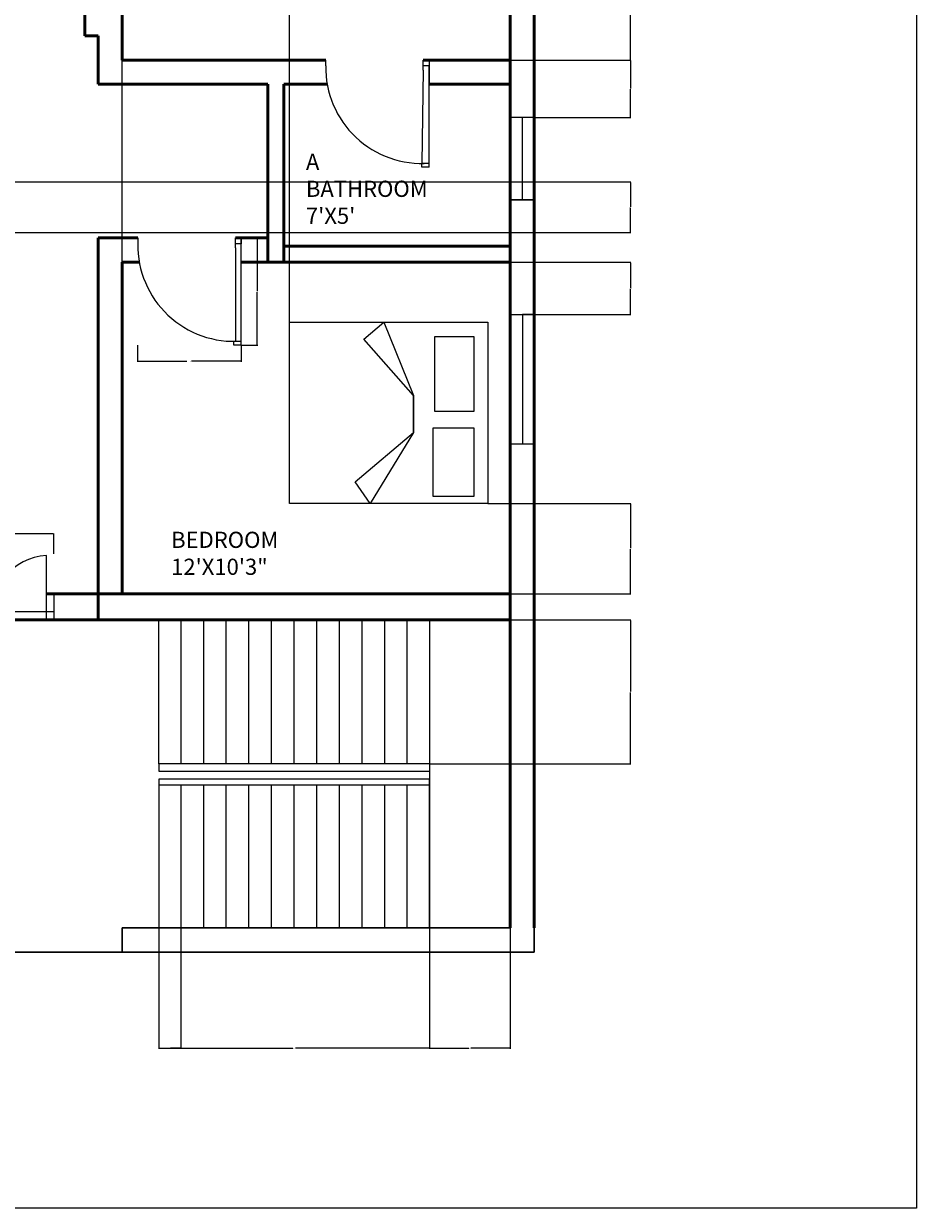
# Model space of a CAD drawing. Units: inches. Extents: x -177 to 2564, y -706 to 2548.
# Tile 2 of 4: x 192 to 523, y -706 to -266. Entities that reach past the tile are written whole.
import ezdxf

# ---------------------------------------------------------------- set-up
doc = ezdxf.new("R2010")
doc.units = ezdxf.units.IN
doc.header["$MEASUREMENT"] = 0
for name, color, linetype, lineweight in [('A-ANNO-DIMS', 2, 'Continuous', 18), ('A-ANNO-TTLB', 7, 'Continuous', 25), ('A-AREA-IDEN', 7, 'Continuous', 25), ('A-DOOR', 3, 'Continuous', 25), ('A-FLOR-OTLN', 7, 'Continuous', 30), ('A-FLOR-STRS', 6, 'Continuous', 25), ('A-FURN', 8, 'Continuous', 18), ('A-GLAZ', 4, 'Continuous', 18), ('A-WALL', 7, 'Continuous', 50)]:
    doc.layers.add(name, color=color, linetype=linetype, lineweight=lineweight)
doc.styles.get("Standard").update_dxf_attribs({"font": 'arial.ttf'})
doc.dimstyles.get("Standard").update_dxf_attribs({"dimtxt": 0.18, "dimasz": 0.18, "dimexe": 0.18, "dimexo": 0.0625, "dimgap": 0.09, "dimtad": 0, "dimtih": 1, "dimtoh": 1, "dimdec": 0, "dimzin": 0, "dimdsep": 46, "dimlunit": 4, "dimtxsty": 'Standard', "dimcen": 0.09, "dimadec": 0, "dimazin": 0, "dimtfac": 1, "dimtdec": 0, "dimtofl": 0, "dimtmove": 0, "dimatfit": 3, "dimfxl": 1, "dimtolj": 1, "dimtzin": 0, "dimarcsym": 0})

# ---------------------------------------------------------------- blocks, each defined once
blk = doc.blocks.new('BED-DOUBLE')
for p, q in [((0, -38.58), (27.19, -27.51)), ((27.19, -27.51), (6.3, -46)), ((27.19, -27.51), (40.92, -27.51)), ((40.92, -27.51), (27.19, -27.51)), ((40.92, -27.51), (67.3, -43.62)), ((59.29, -49.22), (40.92, -27.51)), ((0, -73.65), (0, -38.58)), ((6.3, -46), (0, -38.58)), ((67.3, -43.62), (59.29, -49.22))]:
    blk.add_line(p, q)
for points in [[(0, 0), (67.3, 0), (67.3, -73.65), (0, -73.65)], [(5.32, -5.1), (33.21, -5.1), (33.21, -19.67), (5.32, -19.67)], [(39.24, -5.1), (64.75, -5.1), (64.75, -20.23), (39.24, -20.23)]]:
    blk.add_lwpolyline(points, close=True)
blk = doc.blocks.new('WIN-48')
for p, q in [((0, 0), (9, 0)), ((9, 0), (4.59, 0)), ((4.59, 0), (4.59, -48.06)), ((9, -48.06), (0, -48.06))]:
    blk.add_line(p, q)
blk = doc.blocks.new('WIN-30')
for p, q in [((0, 30.54), (-9, 30.54)), ((-4.41, 0), (-4.41, 30.54)), ((0, 0), (-9, 0)), ((0, 0), (-4.41, 0))]:
    blk.add_line(p, q)
blk = doc.blocks.new('DOOR-SINGLE-36-ALT')
for p, q in [((0, -3.72), (0, 0)), ((0, 0), (2.14, 0)), ((2.14, 0), (2.14, -2.15)), ((-36.24, -2.15), (-36.24, -2.15)), ((-36.24, -2.15), (-36.24, -3.72)), ((-36.24, -3.72), (-36.23, -3.72)), ((2.14, -2.15), (0, -2.15)), ((2.14, -39.77), (2.14, -2.15)), ((-0.59, -39.77), (-0.59, -38.25)), ((-0.59, -38.25), (2.14, -38.25)), ((2.14, -39.77), (-0.59, -39.77))]:
    blk.add_line(p, q)
blk.add_arc((-0.56, -2.67), 35.69, 179.1597, 274.3396)
blk = doc.blocks.new('DOOR-PAIR-44')
for p, q in [((0, 0), (0, 24.32)), ((44.01, 0), (44.01, 23.95)), ((-2.88, 0), (-2.88, 3.11)), ((-2.88, 3.11), (46.72, 3.11)), ((46.72, 0), (-2.88, 0)), ((-2.88, 0), (0, 0)), ((0, 0), (44.01, 0)), ((23.01, 0), (23.01, 3.55)), ((44.01, 0), (23.01, 0)), ((46.72, 0), (44.01, 0))]:
    blk.add_line(p, q)
for centre, radius, start, end in [((0.52, 1.77), 22.55, 355.4915, 91.326), ((45.7, 1.28), 22.73, 94.2755, 183.2347)]:
    blk.add_arc(centre, radius, start, end)
blk = doc.blocks.new('*D18')
at = {"layer": 'A-ANNO-DIMS', "color": 0, "lineweight": -2, "transparency": 16777216}
for p, q in [((272.68, -345.46), (278.76, -345.46)), ((278.58, -345.64), (278.58, -365.17)), ((278.58, -385.05), (278.58, -365.53)), ((272.68, -385.23), (278.76, -385.23))]:
    blk.add_line(p, q, dxfattribs=at)
at = {"layer": 'A-ANNO-DIMS', "color": 0, "transparency": 16777216}
for points in [[(278.55, -345.64), (278.61, -345.64), (278.58, -345.46)], [(278.55, -385.05), (278.61, -385.05), (278.58, -385.23)]]:
    blk.add_solid(points, dxfattribs=at)
at = {"layer": 'Defpoints', "color": 0, "transparency": 16777216}
for p in [(272.61, -345.46), (278.58, -345.46), (272.61, -385.23)]:
    blk.add_point(p, dxfattribs=at)
at = {"layer": 'A-ANNO-DIMS', "color": 0, "transparency": 16777216, "insert": (278.58, -365.35), "char_height": 0.18, "attachment_point": 5}
blk.add_mtext('\\A1;DOOR D2 3\'-4" TYP.', dxfattribs=at)
blk = doc.blocks.new('*D19')
at = {"layer": 'A-ANNO-DIMS', "color": 0, "lineweight": -2, "transparency": 16777216}
for p, q in [((234.08, -385.3), (234.08, -391.38)), ((272.61, -385.3), (272.61, -391.38)), ((234.26, -391.2), (252.5, -391.2)), ((272.43, -391.2), (254.2, -391.2))]:
    blk.add_line(p, q, dxfattribs=at)
at = {"layer": 'A-ANNO-DIMS', "color": 0, "transparency": 16777216}
for points in [[(234.26, -391.17), (234.26, -391.23), (234.08, -391.2)], [(272.43, -391.17), (272.43, -391.23), (272.61, -391.2)]]:
    blk.add_solid(points, dxfattribs=at)
at = {"layer": 'Defpoints', "color": 0, "transparency": 16777216}
for p in [(234.08, -385.23), (272.61, -385.23), (272.61, -391.2)]:
    blk.add_point(p, dxfattribs=at)
at = {"layer": 'A-ANNO-DIMS', "color": 0, "transparency": 16777216, "insert": (253.35, -391.2), "char_height": 0.18, "attachment_point": 5}
blk.add_mtext('\\A1;3\'-2 1/2" TYP.', dxfattribs=at)
blk = doc.blocks.new('*D20')
at = {"layer": 'A-ANNO-DIMS', "color": 0, "lineweight": -2, "transparency": 16777216}
for p, q in [((153.41, -462.66), (153.41, -455.1)), ((153.59, -455.28), (176.76, -455.28)), ((202.83, -455.28), (179.66, -455.28)), ((203.01, -462.66), (203.01, -455.1))]:
    blk.add_line(p, q, dxfattribs=at)
at = {"layer": 'A-ANNO-DIMS', "color": 0, "transparency": 16777216}
for points in [[(153.59, -455.25), (153.59, -455.31), (153.41, -455.28)], [(202.83, -455.25), (202.83, -455.31), (203.01, -455.28)]]:
    blk.add_solid(points, dxfattribs=at)
at = {"layer": 'Defpoints', "color": 0, "transparency": 16777216}
for p in [(203.01, -455.28), (153.41, -462.72), (203.01, -462.72)]:
    blk.add_point(p, dxfattribs=at)
at = {"layer": 'A-ANNO-DIMS', "color": 0, "transparency": 16777216, "insert": (178.21, -455.28), "char_height": 0.18, "attachment_point": 5}
blk.add_mtext('\\A1;DOOR D3 4\'-1 1/2" TYP.', dxfattribs=at)
blk = doc.blocks.new('*D27')
at = {"layer": 'A-ANNO-DIMS', "color": 0, "lineweight": -2, "transparency": 16777216}
for p, q in [((65.01, -324.69), (417.35, -324.69)), ((417.17, -324.87), (417.17, -333.91)), ((417.17, -343.32), (417.17, -334.27)), ((84.12, -343.5), (417.35, -343.5))]:
    blk.add_line(p, q, dxfattribs=at)
at = {"layer": 'A-ANNO-DIMS', "color": 0, "transparency": 16777216}
for points in [[(417.14, -324.87), (417.2, -324.87), (417.17, -324.69)], [(417.14, -343.32), (417.2, -343.32), (417.17, -343.5)]]:
    blk.add_solid(points, dxfattribs=at)
at = {"layer": 'Defpoints', "color": 0, "transparency": 16777216}
for p in [(64.94, -324.69), (84.06, -343.5), (417.17, -343.5)]:
    blk.add_point(p, dxfattribs=at)
at = {"layer": 'A-ANNO-DIMS', "color": 0, "transparency": 16777216, "insert": (417.17, -334.09), "char_height": 0.18, "attachment_point": 5}
blk.add_mtext('\\A1;1\'-7"', dxfattribs=at)
blk = doc.blocks.new('*D40')
at = {"layer": 'A-ANNO-DIMS', "color": 0, "lineweight": -2, "transparency": 16777216}
for p, q in [((242.02, -601.53), (242.02, -646.34)), ((342.59, -601.53), (342.59, -646.34)), ((242.2, -646.16), (291.76, -646.16)), ((342.41, -646.16), (292.84, -646.16))]:
    blk.add_line(p, q, dxfattribs=at)
at = {"layer": 'A-ANNO-DIMS', "color": 0, "transparency": 16777216}
for points in [[(242.2, -646.13), (242.2, -646.19), (242.02, -646.16)], [(342.41, -646.13), (342.41, -646.19), (342.59, -646.16)]]:
    blk.add_solid(points, dxfattribs=at)
at = {"layer": 'Defpoints', "color": 0, "transparency": 16777216}
for p in [(242.02, -601.46), (342.59, -601.46), (342.59, -646.16)]:
    blk.add_point(p, dxfattribs=at)
at = {"layer": 'A-ANNO-DIMS', "color": 0, "transparency": 16777216, "insert": (292.3, -646.16), "char_height": 0.18, "attachment_point": 5}
blk.add_mtext('\\A1;8\'-4 1/2"', dxfattribs=at)
blk = doc.blocks.new('*D41')
at = {"layer": 'A-ANNO-DIMS', "color": 0, "lineweight": -2, "transparency": 16777216}
for p, q in [((342.59, -601.53), (342.59, -646.34)), ((372.47, -601.53), (372.47, -646.34)), ((342.77, -646.16), (357.2, -646.16)), ((372.29, -646.16), (357.86, -646.16))]:
    blk.add_line(p, q, dxfattribs=at)
at = {"layer": 'A-ANNO-DIMS', "color": 0, "transparency": 16777216}
for points in [[(342.77, -646.13), (342.77, -646.19), (342.59, -646.16)], [(372.29, -646.13), (372.29, -646.19), (372.47, -646.16)]]:
    blk.add_solid(points, dxfattribs=at)
at = {"layer": 'Defpoints', "color": 0, "transparency": 16777216}
for p in [(342.59, -601.46), (372.47, -601.46), (372.47, -646.16)]:
    blk.add_point(p, dxfattribs=at)
at = {"layer": 'A-ANNO-DIMS', "color": 0, "transparency": 16777216, "insert": (357.53, -646.16), "char_height": 0.18, "attachment_point": 5}
blk.add_mtext('\\A1;2\'-6"', dxfattribs=at)
blk = doc.blocks.new('*D42')
at = {"layer": 'A-ANNO-DIMS', "color": 0, "lineweight": -2, "transparency": 16777216}
for p, q in [((342.65, -487.19), (417.35, -487.19)), ((417.17, -487.37), (417.17, -513.7)), ((417.17, -540.41), (417.17, -514.07)), ((342.65, -540.59), (417.35, -540.59))]:
    blk.add_line(p, q, dxfattribs=at)
at = {"layer": 'A-ANNO-DIMS', "color": 0, "transparency": 16777216}
for points in [[(417.14, -487.37), (417.2, -487.37), (417.17, -487.19)], [(417.14, -540.41), (417.2, -540.41), (417.17, -540.59)]]:
    blk.add_solid(points, dxfattribs=at)
at = {"layer": 'Defpoints', "color": 0, "transparency": 16777216}
for p in [(342.59, -487.19), (342.59, -540.59), (417.17, -540.59)]:
    blk.add_point(p, dxfattribs=at)
at = {"layer": 'A-ANNO-DIMS', "color": 0, "transparency": 16777216, "insert": (417.17, -513.89), "char_height": 0.18, "attachment_point": 5}
blk.add_mtext('\\A1;4\'-5 1/2"', dxfattribs=at)
blk = doc.blocks.new('*D43')
at = {"layer": 'A-ANNO-DIMS', "color": 0, "lineweight": -2, "transparency": 16777216}
for p, q in [((242.02, -601.53), (242.02, -646.34)), ((250.19, -601.53), (250.19, -646.34)), ((242.2, -646.16), (245.77, -646.16)), ((250.01, -646.16), (246.43, -646.16))]:
    blk.add_line(p, q, dxfattribs=at)
at = {"layer": 'A-ANNO-DIMS', "color": 0, "transparency": 16777216}
for points in [[(242.2, -646.13), (242.2, -646.19), (242.02, -646.16)], [(250.01, -646.13), (250.01, -646.19), (250.19, -646.16)]]:
    blk.add_solid(points, dxfattribs=at)
at = {"layer": 'Defpoints', "color": 0, "transparency": 16777216}
for p in [(242.02, -601.46), (250.19, -601.46), (250.19, -646.16)]:
    blk.add_point(p, dxfattribs=at)
at = {"layer": 'A-ANNO-DIMS', "color": 0, "transparency": 16777216, "insert": (246.1, -646.16), "char_height": 0.18, "attachment_point": 5}
blk.add_mtext('\\A1;0\'-8"', dxfattribs=at)
blk = doc.blocks.new('*D47')
at = {"layer": 'A-ANNO-DIMS', "color": 0, "lineweight": -2, "transparency": 16777216}
for p, q in [((347.99, -206.63), (417.35, -206.63)), ((417.17, -206.81), (417.17, -242.87)), ((417.17, -279.28), (417.17, -243.23)), ((372.54, -279.46), (417.35, -279.46))]:
    blk.add_line(p, q, dxfattribs=at)
at = {"layer": 'A-ANNO-DIMS', "color": 0, "transparency": 16777216}
for points in [[(417.14, -206.81), (417.2, -206.81), (417.17, -206.63)], [(417.14, -279.28), (417.2, -279.28), (417.17, -279.46)]]:
    blk.add_solid(points, dxfattribs=at)
at = {"layer": 'Defpoints', "color": 0, "transparency": 16777216}
for p in [(347.93, -206.63), (417.17, -206.63), (372.47, -279.46)]:
    blk.add_point(p, dxfattribs=at)
at = {"layer": 'A-ANNO-DIMS', "color": 0, "transparency": 16777216, "insert": (417.17, -243.05), "char_height": 0.18, "attachment_point": 5}
blk.add_mtext('\\A1;6\'-1"', dxfattribs=at)
blk = doc.blocks.new('*D48')
at = {"layer": 'A-ANNO-DIMS', "color": 0, "lineweight": -2, "transparency": 16777216}
for p, q in [((228.47, -477.4), (228.47, 71.74)), ((228.65, 71.56), (259.17, 71.56)), ((290.34, 71.56), (259.83, 71.56)), ((290.52, -443.93), (290.52, 71.74))]:
    blk.add_line(p, q, dxfattribs=at)
at = {"layer": 'A-ANNO-DIMS', "color": 0, "transparency": 16777216}
for points in [[(228.65, 71.59), (228.65, 71.53), (228.47, 71.56)], [(290.34, 71.59), (290.34, 71.53), (290.52, 71.56)]]:
    blk.add_solid(points, dxfattribs=at)
at = {"layer": 'Defpoints', "color": 0, "transparency": 16777216}
for p in [(290.52, 71.56), (290.52, -443.99), (228.47, -477.46)]:
    blk.add_point(p, dxfattribs=at)
at = {"layer": 'A-ANNO-DIMS', "color": 0, "transparency": 16777216, "insert": (259.5, 71.56), "char_height": 0.18, "attachment_point": 5}
blk.add_mtext('\\A1;5\'-2"', dxfattribs=at)
blk = doc.blocks.new('*D49')
at = {"layer": 'A-ANNO-DIMS', "color": 0, "lineweight": -2, "transparency": 16777216}
for p, q in [((364.23, -443.99), (417.35, -443.99)), ((417.17, -444.17), (417.17, -460.54)), ((417.17, -477.28), (417.17, -460.91)), ((372.54, -477.46), (417.35, -477.46))]:
    blk.add_line(p, q, dxfattribs=at)
at = {"layer": 'A-ANNO-DIMS', "color": 0, "transparency": 16777216}
for points in [[(417.14, -444.17), (417.2, -444.17), (417.17, -443.99)], [(417.14, -477.28), (417.2, -477.28), (417.17, -477.46)]]:
    blk.add_solid(points, dxfattribs=at)
at = {"layer": 'Defpoints', "color": 0, "transparency": 16777216}
for p in [(364.17, -443.99), (417.17, -443.99), (372.47, -477.46)]:
    blk.add_point(p, dxfattribs=at)
at = {"layer": 'A-ANNO-DIMS', "color": 0, "transparency": 16777216, "insert": (417.17, -460.73), "char_height": 0.18, "attachment_point": 5}
blk.add_mtext('\\A1;2\'-9 1/2"', dxfattribs=at)
blk = doc.blocks.new('*D54')
at = {"layer": 'A-ANNO-DIMS', "color": 0, "lineweight": -2, "transparency": 16777216}
for p, q in [((372.54, -354.46), (417.35, -354.46)), ((417.17, -354.64), (417.17, -363.99)), ((417.17, -373.69), (417.17, -364.35)), ((381.54, -373.87), (417.35, -373.87))]:
    blk.add_line(p, q, dxfattribs=at)
at = {"layer": 'A-ANNO-DIMS', "color": 0, "transparency": 16777216}
for points in [[(417.14, -354.64), (417.2, -354.64), (417.17, -354.46)], [(417.14, -373.69), (417.2, -373.69), (417.17, -373.87)]]:
    blk.add_solid(points, dxfattribs=at)
at = {"layer": 'Defpoints', "color": 0, "transparency": 16777216}
for p in [(372.47, -354.46), (417.17, -354.46), (381.47, -373.87)]:
    blk.add_point(p, dxfattribs=at)
at = {"layer": 'A-ANNO-DIMS', "color": 0, "transparency": 16777216, "insert": (417.17, -364.17), "char_height": 0.18, "attachment_point": 5}
blk.add_mtext('\\A1;1\'-7 1/2"', dxfattribs=at)
blk = doc.blocks.new('*D61')
at = {"layer": 'A-ANNO-DIMS', "color": 0, "lineweight": -2, "transparency": 16777216}
for p, q in [((372.54, -279.46), (417.35, -279.46)), ((417.17, -279.64), (417.17, -289.95)), ((417.17, -300.63), (417.17, -290.32)), ((381.54, -300.81), (417.35, -300.81))]:
    blk.add_line(p, q, dxfattribs=at)
at = {"layer": 'A-ANNO-DIMS', "color": 0, "transparency": 16777216}
for points in [[(417.14, -279.64), (417.2, -279.64), (417.17, -279.46)], [(417.14, -300.63), (417.2, -300.63), (417.17, -300.81)]]:
    blk.add_solid(points, dxfattribs=at)
at = {"layer": 'Defpoints', "color": 0, "transparency": 16777216}
for p in [(372.47, -279.46), (381.47, -300.81), (417.17, -300.81)]:
    blk.add_point(p, dxfattribs=at)
at = {"layer": 'A-ANNO-DIMS', "color": 0, "transparency": 16777216, "insert": (417.17, -290.14), "char_height": 0.18, "attachment_point": 5}
blk.add_mtext('\\A1;1\'-9 1/2"', dxfattribs=at)

msp = doc.modelspace()

# ---------------------------------------------------------------- linework, layer by layer
at = {"layer": 'A-ANNO-TTLB'}
msp.add_lwpolyline([(-176.6, 185.58), (523.32, 185.58), (523.32, -705.52), (-176.6, -705.52)], close=True, dxfattribs=at)
at = {"layer": 'A-DOOR'}
for p, q in [((304.01, -281.61), (304.01, -279.46)), ((340.26, -279.46), (342.4, -279.46)), ((342.4, -279.46), (342.4, -288.46)), ((340.26, -283.18), (339.67, -317.72)), ((234.31, -345.46), (234.23, -347.61)), ((272.61, -354.46), (272.61, -345.46)), ((270.47, -349.18), (270.47, -383.72)), ((203.01, -477.46), (203.01, -487.19))]:
    msp.add_line(p, q, dxfattribs=at)
at = {"layer": 'A-FLOR-OTLN'}
for p, q in [((228.47, -610.46), (228.47, -601.46)), ((228.47, -601.46), (372.47, -601.46)), ((381.47, -601.46), (381.47, -610.46)), ((228.47, -610.46), (3.47, -610.46)), ((381.47, -610.46), (228.47, -610.46))]:
    msp.add_line(p, q, dxfattribs=at)
at = {"layer": 'A-FLOR-STRS'}
for p, q in [((242.02, -540.59), (242.02, -487.19)), ((250.19, -487.19), (250.19, -540.59)), ((258.59, -487.19), (258.59, -540.59)), ((266.99, -487.19), (266.99, -540.59)), ((275.39, -487.19), (275.39, -540.59)), ((283.79, -487.19), (283.79, -540.59)), ((292.19, -487.19), (292.19, -540.59)), ((300.59, -487.19), (300.59, -540.59)), ((308.99, -487.19), (308.99, -540.59)), ((317.39, -487.19), (317.39, -540.59)), ((325.79, -487.19), (325.79, -540.59)), ((342.59, -487.19), (334.19, -487.19)), ((334.19, -487.19), (334.19, -540.59)), ((372.47, -487.19), (342.59, -487.19)), ((342.59, -487.19), (342.59, -601.46)), ((342.59, -487.19), (342.59, -540.59)), ((342.59, -540.59), (242.02, -540.59)), ((242.02, -540.59), (242.02, -543.28)), ((242.02, -543.28), (342.59, -543.28)), ((342.59, -543.28), (342.59, -548.54)), ((342.59, -546.25), (242.02, -546.25)), ((242.02, -546.25), (242.02, -548.54)), ((342.59, -548.54), (242.02, -548.54)), ((242.02, -548.54), (242.02, -601.46)), ((250.19, -548.54), (250.19, -601.46)), ((258.59, -548.54), (258.59, -601.46)), ((266.99, -548.54), (266.99, -601.46)), ((275.39, -548.54), (275.39, -601.46)), ((283.79, -548.54), (283.79, -601.46)), ((292.19, -548.54), (292.19, -601.46)), ((300.59, -548.54), (300.59, -601.46)), ((308.99, -548.54), (308.99, -601.46)), ((317.39, -548.54), (317.39, -601.46)), ((325.79, -548.54), (325.79, -601.46)), ((342.59, -548.54), (334.19, -548.54)), ((334.19, -548.54), (334.19, -601.46)), ((342.59, -548.54), (342.59, -546.25)), ((342.59, -601.46), (342.59, -548.54)), ((342.59, -548.54), (342.59, -548.54))]:
    msp.add_line(p, q, dxfattribs=at)
at = {"layer": 'A-GLAZ'}
for p, q in [((381.47, -331.35), (372.47, -331.35)), ((372.47, -331.35), (381.47, -331.35))]:
    msp.add_line(p, q, dxfattribs=at)
at = {"layer": 'A-WALL'}
for p, q in [((381.47, -601.46), (381.47, 20.54)), ((372.47, 11.54), (372.47, -601.46)), ((228.47, -228.9), (228.47, -279.46)), ((214.58, -270.46), (214.58, -261.46)), ((219.47, -270.46), (214.58, -270.46)), ((219.47, -279.46), (219.47, -270.46)), ((219.47, -279.46), (219.47, -270.46)), ((219.47, -279.46), (219.47, -288.46)), ((228.47, -279.46), (304.01, -279.46)), ((340.26, -279.46), (372.47, -279.46)), ((228.47, -288.46), (219.47, -288.46)), ((228.47, -288.46), (282.47, -288.46)), ((282.47, -288.46), (282.47, -354.46)), ((288.47, -348.46), (288.47, -288.46)), ((288.47, -288.46), (304.57, -288.46)), ((288.47, -288.46), (304.57, -288.46)), ((342.4, -288.46), (372.47, -288.46)), ((372.47, -288.46), (372.47, -348.46)), ((228.47, -345.46), (219.47, -345.46)), ((219.47, -345.46), (219.47, -354.46)), ((228.47, -345.46), (234.31, -345.46)), ((282.47, -345.46), (270.47, -345.46)), ((282.47, -354.46), (282.47, -345.46)), ((372.47, -348.46), (288.47, -348.46)), ((288.47, -354.46), (288.47, -348.46)), ((372.47, -348.46), (372.47, -354.46)), ((219.47, -354.46), (219.47, -478.19)), ((228.47, -354.46), (228.47, -477.46)), ((234.79, -354.46), (228.47, -354.46)), ((372.47, -354.46), (272.61, -354.46)), ((282.47, -354.46), (272.61, -354.46)), ((282.47, -354.46), (288.47, -354.46)), ((372.47, -354.46), (288.47, -354.46)), ((228.47, -477.46), (200.3, -477.46)), ((219.47, -477.46), (203.01, -477.46)), ((219.47, -478.19), (219.47, -487.19)), ((228.47, -477.46), (372.47, -477.46)), ((219.47, -487.19), (3.47, -487.19)), ((203.01, -487.19), (219.47, -487.19)), ((219.47, -487.19), (372.47, -487.19))]:
    msp.add_line(p, q, dxfattribs=at)

# ---------------------------------------------------------------- block references
at = {"layer": 'A-DOOR'}
for name, p in [('DOOR-SINGLE-36-ALT', (340.26, -279.46)), ('DOOR-SINGLE-36-ALT', (270.47, -345.46)), ('DOOR-PAIR-44', (156.29, -487.19))]:
    msp.add_blockref(name, p, dxfattribs=at)
at = {"layer": 'A-FURN', "rotation": 270.0000000000001}
msp.add_blockref('BED-DOUBLE', (364.17, -376.69), dxfattribs=at)
at = {"layer": 'A-GLAZ'}
for name, p in [('WIN-30', (381.47, -331.35)), ('WIN-48', (372.47, -373.87))]:
    msp.add_blockref(name, p, dxfattribs=at)

# ---------------------------------------------------------------- texts
at = {"layer": 'A-AREA-IDEN', "insert": (296.67, -314.23), "char_height": 6, "attachment_point": 1}
msp.add_mtext_dynamic_manual_height_columns("A BATHROOM\\P7'X5'", width=0.4581, gutter_width=1, heights=[0], dxfattribs=at)
at = {"layer": 'A-AREA-IDEN', "insert": (246.62, -454.48), "char_height": 6, "attachment_point": 1}
msp.add_mtext('BEDROOM\\P12\'X10\'3"', dxfattribs=at)

# ---------------------------------------------------------------- dimensions: what is measured, and where the dimension line sits
at = {"layer": 'A-ANNO-DIMS'}
for base, p1, p2, picture, middle in [((290.52, 71.5552), (228.4733, -477.4645), (290.52, -443.9906), '*D48', (259.4967, 71.5552)), ((342.59, -646.16), (242.02, -601.46), (342.59, -601.46), '*D40', (292.3, -646.16)), ((250.19, -646.16), (242.02, -601.46), (250.19, -601.46), '*D43', (246.1, -646.16)), ((372.47, -646.16), (342.59, -601.46), (372.47, -601.46), '*D41', (357.53, -646.16))]:
    dim = msp.add_linear_dim(base=base, p1=p1, p2=p2, dimstyle='Standard', override={"dimdec": 1, "dimlfac": 1, "dimrnd": 0, "dimzin": 1, "dimdsep": 46, "dimlunit": 4, "dimfrac": 2}, dxfattribs=at)
    dim.commit()
    dim.dimension.update_dxf_attribs({"geometry": picture, "text_midpoint": middle})
for base, p1, p2, picture, middle in [((417.17, -206.63), (372.47, -279.46), (347.93, -206.63), '*D47', (417.17, -243.05)), ((417.1733, -300.8116), (372.4733, -279.4645), (381.4733, -300.8116), '*D61', (417.1733, -290.138)), ((417.17, -343.5), (64.94, -324.69), (84.06, -343.5), '*D27', (417.17, -334.09)), ((417.17, -354.46), (381.47, -373.87), (372.47, -354.46), '*D54', (417.17, -364.17)), ((417.17, -443.99), (372.47, -477.46), (364.17, -443.99), '*D49', (417.17, -460.73)), ((417.17, -540.59), (342.59, -487.19), (342.59, -540.59), '*D42', (417.17, -513.89))]:
    dim = msp.add_linear_dim(base=base, p1=p1, p2=p2, angle=90, dimstyle='Standard', override={"dimdec": 1, "dimlfac": 1, "dimrnd": 0, "dimzin": 1, "dimdsep": 46, "dimlunit": 4, "dimfrac": 2}, dxfattribs=at)
    dim.commit()
    dim.dimension.update_dxf_attribs({"geometry": picture, "text_midpoint": middle})
dim = msp.add_linear_dim(base=(278.58, -345.46), p1=(272.61, -385.23), p2=(272.61, -345.46), angle=90, text='DOOR D2 <> TYP.', dimstyle='Standard', override={"dimdec": 1, "dimlfac": 1, "dimrnd": 0, "dimzin": 1, "dimdsep": 46, "dimlunit": 4, "dimfrac": 2}, dxfattribs=at)
dim.commit()
dim.dimension.update_dxf_attribs({"geometry": '*D18', "text_midpoint": (278.58, -365.35)})
for base, p1, p2, text, picture, middle in [((272.61, -391.2), (234.08, -385.23), (272.61, -385.23), '<> TYP.', '*D19', (253.35, -391.2)), ((203.01, -455.28), (153.41, -462.72), (203.01, -462.72), 'DOOR D3 <> TYP.', '*D20', (178.21, -455.28))]:
    dim = msp.add_linear_dim(base=base, p1=p1, p2=p2, text=text, dimstyle='Standard', override={"dimdec": 1, "dimlfac": 1, "dimrnd": 0, "dimzin": 1, "dimdsep": 46, "dimlunit": 4, "dimfrac": 2}, dxfattribs=at)
    dim.commit()
    dim.dimension.update_dxf_attribs({"geometry": picture, "text_midpoint": middle})

doc.saveas('drawing.dxf')
